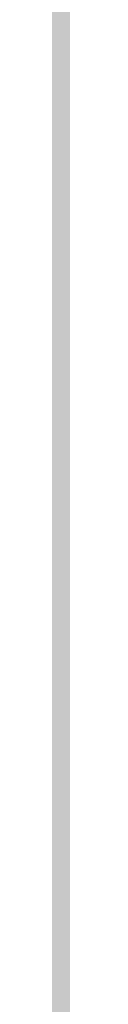
# Model space of a CAD drawing. Units: inches. Extents: x 2083 to 3317, y 1141 to 2115.
# Tile 218 of 256: x 3126.939 to 3126.956, y 1265.165 to 1267.234. Entities that reach past the tile are written whole.
import ezdxf

# ---------------------------------------------------------------- set-up
doc = ezdxf.new("R2010")
doc.units = ezdxf.units.IN
doc.layers.add('A-ANNO-DIMS', color=2, linetype='Continuous', lineweight=18)
doc.layers.add('A-WALL-PATT', color=251, linetype='Continuous', lineweight=13, true_color=0x636466)
doc.styles.get("Standard").update_dxf_attribs({"font": 'arial.ttf'})
doc.dimstyles.new('ISO-25', dxfattribs={"dimtxt": 12, "dimasz": 12, "dimexe": 1.25, "dimexo": 0.625, "dimtad": 1, "dimlunit": 3, "dimtxsty": 'Standard', "dimcen": 2.5, "dimadec": 0, "dimazin": 0, "dimtfac": 1, "dimtmove": 0, "dimatfit": 3, "dimfxl": 1, "dimarcsym": 0})

# ---------------------------------------------------------------- blocks, each defined once
blk = doc.blocks.new('*D26')
at = {"layer": 'A-ANNO-DIMS', "color": 0, "lineweight": -2, "transparency": 16777216}
for p, q in [((3088.9858, 1274.9151), (3088.9858, 1270.952)), ((3111.24, 1274.9151), (3111.24, 1270.952)), ((3076.9858, 1272.202), (2840.2624, 1272.202)), ((3111.24, 1272.202), (3088.9858, 1272.202)), ((3123.24, 1272.202), (3135.24, 1272.202))]:
    blk.add_line(p, q, dxfattribs=at)
at = {"layer": 'A-ANNO-DIMS', "color": 0, "transparency": 16777216}
for points in [[(3076.9858, 1274.202), (3076.9858, 1270.202), (3088.9858, 1272.202)], [(3123.24, 1274.202), (3123.24, 1270.202), (3111.24, 1272.202)]]:
    blk.add_solid(points, dxfattribs=at)
at = {"layer": 'Defpoints', "color": 0, "transparency": 16777216}
for p in [(3088.9858, 1275.5401), (3111.24, 1275.5401), (3088.9858, 1272.202)]:
    blk.add_point(p, dxfattribs=at)
at = {"layer": 'A-ANNO-DIMS', "color": 0, "transparency": 16777216, "insert": (2952.6241, 1279.0316), "char_height": 12, "attachment_point": 5}
blk.add_mtext('NIGHTSTAND 1\'-10 1/2" TYP.', dxfattribs=at)
blk = doc.blocks.new('*D27')
at = {"layer": 'A-ANNO-DIMS', "color": 0, "lineweight": -2, "transparency": 16777216}
for p, q in [((3114.5782, 1309.7943), (3114.5782, 1321.7943)), ((3111.865, 1297.7943), (3115.8282, 1297.7943)), ((3114.5782, 1297.7943), (3114.5782, 1275.5401)), ((3111.865, 1275.5401), (3115.8282, 1275.5401)), ((3114.5782, 1263.5401), (3114.5782, 1140.9886))]:
    blk.add_line(p, q, dxfattribs=at)
at = {"layer": 'A-ANNO-DIMS', "color": 0, "transparency": 16777216}
for points in [[(3112.5782, 1309.7943), (3116.5782, 1309.7943), (3114.5782, 1297.7943)], [(3112.5782, 1263.5401), (3116.5782, 1263.5401), (3114.5782, 1275.5401)]]:
    blk.add_solid(points, dxfattribs=at)
at = {"layer": 'Defpoints', "color": 0, "transparency": 16777216}
for p in [(3111.24, 1297.7943), (3111.24, 1275.5401), (3114.5782, 1275.5401)]:
    blk.add_point(p, dxfattribs=at)
at = {"layer": 'A-ANNO-DIMS', "color": 0, "transparency": 16777216, "insert": (3107.7485, 1196.2643), "char_height": 12, "attachment_point": 5, "rotation": 90}
blk.add_mtext('1\'-10 1/2" TYP.', dxfattribs=at)

msp = doc.modelspace()

# ---------------------------------------------------------------- hatches: boundary and pattern name
at = {"layer": 'A-WALL-PATT'}
h = msp.add_hatch(color=256, dxfattribs=at)
h.dxf.hatch_style = 1
h.paths.add_polyline_path([(3126.9598, 2020.7614), (2748.9598, 2020.7614), (2604.9598, 2020.7614), (2226.9598, 2020.7614), (2226.9598, 1702.7614), (2466.9598, 1702.7614), (2466.9598, 1582.7614), (2418.9598, 1582.7614), (2418.9598, 1477.7614), (2226.9598, 1477.7614), (2226.9598, 1263.2614), (2544.9598, 1263.2614), (2544.9598, 1411.7614), (2604.9598, 1411.7614), (2685.9598, 1411.7614), (2685.9598, 1420.7614), (2604.9598, 1420.7614), (2604.9598, 1573.7614), (2604.9598, 1702.7614), (2604.9598, 2011.7614), (2748.9598, 2011.7614), (2748.9598, 1702.7614), (2862.9598, 1702.7614), (2862.9598, 1621.7614), (2871.9598, 1621.7614), (2871.9598, 1702.7614), (2883.9598, 1702.7614), (2883.9598, 1706.9395, -0.026459), (2883.9598, 1711.7614), (2757.9598, 1711.7614), (2757.9598, 1807.7614), (2787.9598, 1807.7614), (2787.9598, 1812.2614), (2757.9598, 1812.2614), (2757.9598, 2011.7614), (2877.9598, 2011.7614), (2877.9598, 1812.2614), (2847.9598, 1812.2614), (2847.9598, 1807.7614), (2889.8357, 1807.7614), (2889.8357, 1812.2614), (2882.4598, 1812.2614), (2882.4598, 2011.7614), (3117.9598, 2011.7614), (3117.9598, 1812.2614), (2937.8357, 1812.2614), (2937.8357, 1807.7614), (2995.7098, 1807.7614), (2995.7098, 1796.1177), (3000.2098, 1796.1177), (3000.2098, 1807.7614), (3117.9598, 1807.7614), (3117.9598, 1711.7614), (3000.2098, 1711.7614), (3000.2098, 1760.1177), (2998.5727, 1760.1177, -0.020711), (2995.7098, 1760.1177), (2995.7098, 1711.7614), (2931.9598, 1711.7614), (2931.9598, 1702.7614), (3126.9598, 1702.7614)])
h.paths.add_polyline_path([(2471.4598, 2011.7614), (2471.4598, 1810.0114), (2462.7169, 1810.0114), (2462.7169, 1805.5114), (2505.9598, 1805.5114), (2505.9598, 1810.0114), (2475.9598, 1810.0114), (2475.9598, 2011.7614), (2595.9598, 2011.7614), (2595.9598, 1810.0114), (2565.9598, 1810.0114), (2565.9598, 1805.5114), (2595.9598, 1805.5114), (2595.9598, 1711.7614), (2235.9598, 1711.7614), (2235.9598, 1805.5114), (2353.7098, 1805.5114), (2353.7098, 1796.0542), (2358.2098, 1796.0542), (2358.2098, 1805.5114), (2414.7169, 1805.5114), (2414.7169, 1810.0114), (2235.9598, 1810.0114), (2235.9598, 2011.7614)], flags=16)
h.paths.add_polyline_path([(2270.2047, 1994.61), (2270.2047, 1970.61), (2246.2047, 1970.61), (2246.2047, 1994.61)], flags=0)
edge = h.paths.add_edge_path(flags=0)
edge.add_ellipse((2332.0274, 1899.7982), major_axis=(-3.043, 3.043), ratio=0.168252, start_angle=-161.3322, end_angle=-156.3071, ccw=False)
edge.add_ellipse((2333.082, 1898.7435), major_axis=(-1.0546, 1.0546), ratio=0.453532, start_angle=-123.371, end_angle=-94.1591)
edge = h.paths.add_edge_path(flags=0)
edge.add_ellipse((2332.0274, 1968.8763), major_axis=(3.043, 3.043), ratio=0.168252, start_angle=18.6678, end_angle=23.6929)
edge.add_spline(control_points=[(2332.9256, 1970.6911), (2332.2268, 1970.3361), (2330.8937, 1969.6589), (2328.4131, 1970.9321), (2327.2039, 1967.7487), (2324.7096, 1969.9556), (2322.5328, 1967.0124), (2320.0128, 1971.2958), (2317.6803, 1968.1578), (2316.0405, 1967.102), (2315.4269, 1966.8096)], knot_values=[0, 0, 0, 0, 2.267059, 4.324559, 6.685584, 8.878641, 11.121502, 14.300359, 17.755284, 19.732645, 19.732645, 19.732645, 19.732645], degree=3, periodic=0)
edge.add_ellipse((2332.0274, 1968.8763), major_axis=(3.043, 3.043), ratio=0.168252, start_angle=18.6678, end_angle=23.6929, ccw=False)
edge.add_ellipse((2333.082, 1969.9309), major_axis=(1.0546, 1.0546), ratio=0.453532, start_angle=56.629, end_angle=85.8409, ccw=False)
edge = h.paths.add_edge_path(flags=0)
edge.add_spline(control_points=[(2296.4283, 1967.9879), (2293.6278, 1965.3363), (2287.7036, 1959.7271), (2299.7439, 1949.9957), (2294.5326, 1935.6685), (2290.5732, 1920.6035), (2293.3941, 1909.9737), (2296.1854, 1904.9665)], knot_values=[0.099185, 0.099185, 0.099185, 0.099185, 0.345301, 0.619822, 0.982653, 1.386093, 1.810555, 1.810555, 1.810555, 1.810555], degree=3, periodic=0)
edge.add_spline(control_points=[(2296.1854, 1904.9665), (2297.3836, 1902.6193), (2298.001, 1901.9493), (2298.553, 1901.4682)], knot_values=[0.006246, 0.006246, 0.006246, 0.006246, 0.055476, 0.055476, 0.055476, 0.055476], degree=3, periodic=0)
edge.add_spline(control_points=[(2298.553, 1901.4682), (2297.2586, 1900.9232), (2295.2253, 1900.2321), (2293.0602, 1900.6142), (2292.1014, 1900.7884), (2292.0896, 1900.7906)], knot_values=[0.312835, 0.312835, 0.312835, 0.312835, 0.40178, 0.474987, 0.475903, 0.475903, 0.475903, 0.475903], degree=3, periodic=0)
edge.add_arc((2292.7936, 1904.6641), 3.937, 215.4209, 259.6982, ccw=False)
edge.add_spline(control_points=[(2289.5853, 1902.3823), (2289.4767, 1902.5351), (2289.3685, 1902.688), (2289.2609, 1902.8412)], knot_values=[0.102872, 0.102872, 0.102872, 0.102872, 0.116896, 0.116896, 0.116896, 0.116896], degree=3, periodic=0)
edge.add_spline(control_points=[(2289.2609, 1902.8412), (2288.6866, 1902.5502), (2287.64, 1902.0199), (2285.8813, 1901.874), (2283.853, 1901.5044), (2281.72, 1899.7105), (2278.467, 1899.4929), (2276.1571, 1901.8832), (2272.259, 1899.8041), (2267.7776, 1901.8432), (2262.2439, 1900.184), (2257.4149, 1901.7821), (2254.3184, 1900.7261), (2253.1783, 1900.3373)], knot_values=[0, 0, 0, 0, 1.907977, 3.477176, 5.261074, 7.972851, 11.680248, 13.717921, 16.939592, 22.789562, 27.502503, 33.595215, 37.145618, 37.145618, 37.145618, 37.145618], degree=3, periodic=0)
edge.add_line((2253.1783, 1900.3373), (2250.2442, 1902.8412))
edge.add_line((2250.2442, 1902.8412), (2250.2442, 1965.8333))
edge.add_line((2250.2442, 1965.8333), (2253.1783, 1968.3371))
edge.add_spline(control_points=[(2253.1783, 1968.3371), (2254.3184, 1967.9483), (2257.4149, 1966.8924), (2262.2439, 1968.4904), (2267.7776, 1966.8313), (2271.5267, 1968.5372), (2273.8759, 1967.8283), (2274.2067, 1967.7276)], knot_values=[0, 0, 0, 0, 0.09018, 0.244935, 0.364644, 0.513233, 0.537855, 0.537855, 0.537855, 0.537855], degree=3, periodic=0)
edge.add_arc((2274.3529, 1963.7933), 3.937, 72.0511, 92.1279, ccw=False)
edge.add_arc((2281.2969, 1985.23), 18.5963, 252.05113, 288.56572)
edge.add_arc((2292.3167, 1956.0289), 12.6461, 71.02679, 113.77822, ccw=False)
edge = h.paths.add_edge_path(flags=0)
edge.add_spline(control_points=[(2274.8994, 1951.8562), (2275.0662, 1951.6166), (2275.2327, 1951.3766), (2275.398, 1951.1359)], knot_values=[1.409916, 1.409916, 1.409916, 1.409916, 1.43159, 1.43159, 1.43159, 1.43159], degree=3, periodic=0)
edge.add_spline(control_points=[(2275.398, 1951.1359), (2275.7921, 1950.5619), (2276.1792, 1949.9838), (2276.5455, 1949.3971)], knot_values=[1.358238, 1.358238, 1.358238, 1.358238, 1.409916, 1.409916, 1.409916, 1.409916], degree=3, periodic=0)
edge.add_line((2276.5455, 1949.3971), (2277.4373, 1947.8622))
edge.add_spline(control_points=[(2277.4373, 1947.8622), (2276.3038, 1945.6731), (2274.6397, 1942.4269), (2274.6316, 1938.0939), (2272.7991, 1930.8515), (2274.3564, 1943.897), (2275.9477, 1947.9234), (2276.5455, 1949.3971)], knot_values=[0.005632, 0.005632, 0.005632, 0.005632, 0.186014, 0.266002, 0.357087, 0.59639, 0.739732, 0.739732, 0.739732, 0.739732], degree=3, periodic=0)
edge.add_spline(control_points=[(2276.5455, 1949.3971), (2276.1792, 1949.9838), (2275.7921, 1950.5619), (2275.398, 1951.1359)], knot_values=[1.358238, 1.358238, 1.358238, 1.358238, 1.409916, 1.409916, 1.409916, 1.409916], degree=3, periodic=0)
edge.add_spline(control_points=[(2275.398, 1951.1359), (2274.9425, 1950.0805), (2274.2078, 1948.0253), (2273.9346, 1944.8515), (2272.4685, 1937.6275), (2273.4662, 1945.6965), (2274.7006, 1951.0595), (2274.8994, 1951.8562)], knot_values=[0.104364, 0.104364, 0.104364, 0.104364, 0.189636, 0.269624, 0.36071, 0.600013, 0.644622, 0.644622, 0.644622, 0.644622], degree=3, periodic=0)
h.paths.add_polyline_path([(2269.1675, 1963.1276, -0.357527), (2268.1706, 1960.9764, -0.092561), (2268.1706, 1939.4363, -0.357527), (2269.1675, 1937.2851, -0.357527), (2267.0163, 1938.282, -0.164785), (2254.6856, 1938.282, -0.357527), (2252.5344, 1937.2851, -0.357527), (2253.5313, 1939.4363, -0.092561), (2253.5313, 1960.9764, -0.357527), (2252.5344, 1963.1276, -0.357527), (2254.6856, 1962.1307, -0.164785), (2267.0163, 1962.1307, -0.357527)], flags=0)
h.paths.add_polyline_path([(2248.8741, 1967.8018), (2248.8741, 1957.0277), (2249.4578, 1957.0277), (2249.4578, 1911.6468), (2248.8741, 1911.6468), (2248.8741, 1900.8727), (2246.5119, 1900.8727, 0.197327), (2244.1497, 1902.4569), (2244.1497, 1966.2176, 0.197327), (2246.5119, 1967.8018)], flags=0)
h.paths.add_polyline_path([(2269.1675, 1931.3893, -0.357527), (2268.1706, 1929.2381, -0.092561), (2268.1706, 1907.6981, -0.357527), (2269.1675, 1905.5469, -0.357527), (2267.0163, 1906.5438, -0.164785), (2254.6856, 1906.5438, -0.357527), (2252.5344, 1905.5469, -0.357527), (2253.5313, 1907.6981, -0.092561), (2253.5313, 1929.2381, -0.357527), (2252.5344, 1931.3893, -0.357527), (2254.6856, 1930.3925, -0.164785), (2267.0163, 1930.3925, -0.357527)], flags=0)
edge = h.paths.add_edge_path(flags=0)
edge.add_spline(control_points=[(2276.1969, 1906.7237), (2276.1681, 1909.0289), (2276.114, 1913.3719), (2270.5984, 1924.925), (2273.9052, 1919.0128), (2275.9217, 1916.2621), (2275.4746, 1912.4021), (2277.2579, 1910.3806), (2276.696, 1908.225), (2276.6462, 1906.813), (2276.6178, 1906.0084)], knot_values=[0, 0, 0, 0, 8.61026, 16.221274, 18.843057, 23.804898, 27.440828, 29.356102, 31.203478, 33.650687, 33.650687, 33.650687, 33.650687], degree=3, periodic=0)
edge.add_spline(control_points=[(2276.6178, 1906.0084), (2276.6233, 1905.6241), (2276.4977, 1904.6287), (2275.4418, 1903.8547), (2274.9373, 1903.0804), (2274.8591, 1902.8412)], knot_values=[0.156488, 0.156488, 0.156488, 0.156488, 0.184398, 0.231376, 0.250598, 0.250598, 0.250598, 0.250598], degree=3, periodic=0)
edge.add_line((2274.8591, 1902.8412), (2276.506, 1902.8412))
edge.add_spline(control_points=[(2276.506, 1902.8412), (2276.7883, 1903.0849), (2277.6651, 1904.1252), (2278.2495, 1904.3407), (2277.6539, 1908.5274), (2278.1557, 1906.2278), (2278.1005, 1905.2859), (2278.8467, 1904.069), (2277.8568, 1903.4149), (2277.8742, 1902.991), (2277.9036, 1902.8412)], knot_values=[0.059574, 0.059574, 0.059574, 0.059574, 0.080753, 0.103741, 0.16972, 0.176036, 0.207137, 0.240474, 0.262341, 0.27366, 0.27366, 0.27366, 0.27366], degree=3, periodic=0)
edge.add_line((2277.9036, 1902.8412), (2280.0298, 1902.8412))
edge.add_spline(control_points=[(2280.0298, 1902.8412), (2279.8882, 1903.0884), (2279.4993, 1903.9816), (2280.1523, 1905.9393), (2278.1036, 1909.6578), (2279.7624, 1907.1853), (2280.3279, 1904.8749), (2280.4851, 1903.4896), (2281.4633, 1903.2494), (2281.7583, 1902.9365), (2281.834, 1902.8412)], knot_values=[0.013856, 0.013856, 0.013856, 0.013856, 0.034874, 0.088867, 0.107879, 0.126738, 0.158714, 0.193757, 0.217487, 0.226722, 0.226722, 0.226722, 0.226722], degree=3, periodic=0)
edge.add_spline(control_points=[(2281.834, 1902.8412), (2281.7875, 1902.8267), (2281.647, 1902.783), (2281.3955, 1902.8595), (2281.0881, 1902.9852), (2280.7207, 1903.0609), (2280.3335, 1903.0257), (2280.1248, 1902.8989), (2280.0298, 1902.8412)], knot_values=[0, 0, 0, 0, 0.14413, 0.435517, 0.749276, 1.153046, 1.548371, 1.878348, 1.878348, 1.878348, 1.878348], degree=3, periodic=0)
edge.add_line((2280.0298, 1902.8412), (2277.9036, 1902.8412))
edge.add_spline(control_points=[(2277.9036, 1902.8412), (2277.8929, 1902.7959), (2277.8654, 1902.6796), (2277.6075, 1902.6875), (2277.2741, 1902.8007), (2276.8379, 1902.6198), (2276.5838, 1902.7893), (2276.506, 1902.8412)], knot_values=[0, 0, 0, 0, 0.127189, 0.326199, 0.628009, 1.24357, 1.515331, 1.515331, 1.515331, 1.515331], degree=3, periodic=0)
edge.add_line((2276.506, 1902.8412), (2274.8591, 1902.8412))
edge.add_spline(control_points=[(2274.8591, 1902.8412), (2274.8144, 1902.8986), (2274.7251, 1903.0134), (2274.4935, 1903.119), (2274.2443, 1902.9605), (2273.9371, 1903.1849), (2273.614, 1902.9831), (2273.4083, 1902.883), (2273.3223, 1902.8412)], knot_values=[0, 0, 0, 0, 0.21843, 0.436957, 0.687977, 0.990379, 1.398396, 1.69185, 1.69185, 1.69185, 1.69185], degree=3, periodic=0)
edge.add_spline(control_points=[(2273.3223, 1902.8412), (2273.6167, 1903.4457), (2274.274, 1904.5383), (2276.0272, 1904.5737), (2276.207, 1906.5836), (2276.1969, 1906.7237)], knot_values=[0.012227, 0.012227, 0.012227, 0.012227, 0.059472, 0.106218, 0.134458, 0.134458, 0.134458, 0.134458], degree=3, periodic=0)
h.paths.add_polyline_path([(2270.7761, 1897.7898), (2270.7761, 1873.7898), (2246.7761, 1873.7898), (2246.7761, 1897.7898)], flags=0)
h.paths.add_polyline_path([(2353.7098, 1760.0051), (2353.7098, 1760.0542), (2358.2098, 1760.0542, -0.033729)], flags=0)
h.paths.add_polyline_path([(2321.8191, 1737.5292), (2341.9953, 1737.5292, -0.414214), (2343.2033, 1736.3212), (2343.2033, 1721.0206, -0.414214), (2341.9953, 1719.8127), (2321.8191, 1719.8127, -0.414214), (2320.6112, 1721.0206), (2320.6112, 1736.3212, -0.414214)], flags=0)
h.paths.add_polyline_path([(2324.235, 1736.3212), (2339.5794, 1736.3212, -0.414214), (2341.9953, 1733.9053), (2341.9953, 1725.4497, -0.414214), (2339.5794, 1723.0338), (2333.6806, 1723.0338), (2333.8453, 1722.0455, -0.870646), (2335.4254, 1721.8259, -0.767327), (2333.9227, 1721.4232), (2331.291, 1721.4232, -0.767327), (2329.7883, 1721.8259, -0.870646), (2331.3684, 1722.0455), (2331.5331, 1723.0338), (2324.235, 1723.0338, -0.414214), (2321.8191, 1725.4497), (2321.8191, 1733.9053, -0.414214)], flags=0)
h.paths.add_polyline_path([(2570.4838, 1928.6154), (2589.6838, 1928.6154), (2590.1688, 1928.6154), (2590.1688, 1904.9934), (2570.4838, 1904.9934)], flags=0)
h.paths.add_polyline_path([(2574.4473, 1927.2638, -1), (2572.8288, 1927.2638, -1)], flags=0)
h.paths.add_polyline_path([(2573.0899, 1926.9409), (2573.925, 1927.776), (2574.1477, 1927.5533), (2573.3126, 1926.7182)], flags=0)
h.paths.add_polyline_path([(2578.7791, 1919.7296, -1), (2571.5917, 1919.7296, -1)], flags=0)
h.paths.add_polyline_path([(2578.3854, 1919.7296, -1), (2571.9854, 1919.7296, -1)], flags=0)
h.paths.add_polyline_path([(2331.5958, 1729.4762, -1), (2333.618, 1729.4762, -1)], flags=0)
h.paths.add_polyline_path([(2578.0342, 1927.2638, -1), (2576.4157, 1927.2638, -1)], flags=0)
h.paths.add_polyline_path([(2576.6889, 1927.5311), (2576.9116, 1927.7538), (2577.7467, 1926.9186), (2577.524, 1926.6959)], flags=0)
h.paths.add_polyline_path([(2578.1391, 1909.8595, -1), (2572.2317, 1909.8595, -1)], flags=0)
h.paths.add_polyline_path([(2577.7454, 1909.8595, -1), (2572.6254, 1909.8595, -1)], flags=0)
h.paths.add_polyline_path([(2583.7977, 1927.2638, -1), (2582.1792, 1927.2638, -1)], flags=0)
h.paths.add_polyline_path([(2582.7186, 1927.7538), (2583.5538, 1926.9186), (2583.3311, 1926.6959), (2582.4959, 1927.5311)], flags=0)
h.paths.add_polyline_path([(2582.4959, 1927.5311), (2582.7186, 1927.7538), (2583.5538, 1926.9186), (2583.3311, 1926.6959)], flags=0)
h.paths.add_polyline_path([(2587.7391, 1920.5296, -1), (2581.8317, 1920.5296, -1)], flags=0)
h.paths.add_polyline_path([(2587.3454, 1920.5296, -1), (2582.2254, 1920.5296, -1)], flags=0)
h.paths.add_polyline_path([(2587.3846, 1927.2638, -1), (2585.7661, 1927.2638, -1)], flags=0)
h.paths.add_polyline_path([(2586.082, 1926.9802), (2586.9172, 1927.8154), (2587.1399, 1927.5927), (2586.3047, 1926.7575)], flags=0)
h.paths.add_polyline_path([(2588.3791, 1910.6595, -1), (2581.1917, 1910.6595, -1)], flags=0)
h.paths.add_polyline_path([(2587.9854, 1910.6595, -1), (2581.5854, 1910.6595, -1)], flags=0)
h.paths.add_polyline_path([(2417.1677, 1729.4779), (2437.3439, 1729.4779, -0.414214), (2438.5519, 1728.2699), (2438.5519, 1712.9693, -0.414214), (2437.3439, 1711.7614), (2417.1677, 1711.7614, -0.414214), (2415.9598, 1712.9693), (2415.9598, 1728.2699, -0.414214)], flags=0)
h.paths.add_polyline_path([(2419.5836, 1728.2699), (2434.928, 1728.2699, -0.414214), (2437.3439, 1725.8541), (2437.3439, 1717.3984, -0.414214), (2434.928, 1714.9825), (2429.0292, 1714.9825), (2429.1939, 1713.9942, -0.870646), (2430.774, 1713.7746, -0.767327), (2429.2713, 1713.372), (2426.6396, 1713.372, -0.767327), (2425.1369, 1713.7746, -0.870646), (2426.717, 1713.9942), (2426.8817, 1714.9825), (2419.5836, 1714.9825, -0.414214), (2417.1677, 1717.3984), (2417.1677, 1725.8541, -0.414214)], flags=0)
h.paths.add_polyline_path([(2419.5836, 1728.2699), (2434.928, 1728.2699, -0.414214), (2437.3439, 1725.8541), (2437.3439, 1717.3984, -0.414214), (2434.928, 1714.9825), (2429.0292, 1714.9825), (2428.3581, 1719.009), (2427.5528, 1719.009), (2426.8817, 1714.9825), (2419.5836, 1714.9825, -0.414214), (2417.1677, 1717.3984), (2417.1677, 1725.8541, -0.414214)], flags=0)
h.paths.add_polyline_path([(2426.9444, 1721.4249, -1), (2428.9666, 1721.4249, -1)], flags=0)
h.paths.add_polyline_path([(2475.9598, 1702.7614), (2595.9598, 1702.7614), (2595.9598, 1582.7614), (2475.9598, 1582.7614)], flags=16)
h.paths.add_polyline_path([(2427.9598, 1573.7614), (2595.9598, 1573.7614), (2595.9598, 1468.7614), (2595.9598, 1420.7614), (2384.4598, 1420.7614), (2384.4598, 1468.7614), (2427.9598, 1468.7614)], flags=16)
h.paths.add_polyline_path([(2379.9598, 1468.7614), (2379.9598, 1420.7614), (2235.9598, 1420.7614), (2235.9598, 1468.7614)], flags=16)
h.paths.add_polyline_path([(2317.816, 1466.6958), (2337.9922, 1466.6958, -0.414214), (2339.2002, 1465.4878), (2339.2002, 1450.1872, -0.414214), (2337.9922, 1448.9792), (2317.816, 1448.9792, -0.414214), (2316.6081, 1450.1872), (2316.6081, 1465.4878, -0.414214)], flags=0)
h.paths.add_polyline_path([(2320.2319, 1465.4878), (2335.5763, 1465.4878, -0.414214), (2337.9922, 1463.0719), (2337.9922, 1454.6163, -0.414214), (2335.5763, 1452.2004), (2329.6775, 1452.2004), (2329.8422, 1451.212, -0.870646), (2331.4223, 1450.9925, -0.767327), (2329.9196, 1450.5898), (2327.2879, 1450.5898, -0.767327), (2325.7852, 1450.9925, -0.870646), (2327.3653, 1451.212), (2327.53, 1452.2004), (2320.2319, 1452.2004, -0.414214), (2317.816, 1454.6163), (2317.816, 1463.0719, -0.414214)], flags=0)
h.paths.add_polyline_path([(2320.2319, 1465.4878), (2335.5763, 1465.4878, -0.414214), (2337.9922, 1463.0719), (2337.9922, 1454.6163, -0.414214), (2335.5763, 1452.2004), (2329.6775, 1452.2004), (2329.0064, 1456.2269), (2328.2011, 1456.2269), (2327.53, 1452.2004), (2320.2319, 1452.2004, -0.414214), (2317.816, 1454.6163), (2317.816, 1463.0719, -0.414214)], flags=0)
h.paths.add_polyline_path([(2327.5926, 1458.6428, -1), (2329.6148, 1458.6428, -1)], flags=0)
h.paths.add_polyline_path([(2244.4117, 1433.3405), (2241.9209, 1433.3405, -0.414214), (2240.0179, 1435.2435), (2240.0179, 1440.9528, -0.414211), (2241.9209, 1442.8559), (2244.4117, 1442.8559, -1.976472)], flags=0)
h.paths.add_polyline_path([(2245.3569, 1434.3975, -0.414214), (2245.3569, 1441.7988, -2.144098)], flags=0)
h.paths.add_polyline_path([(2535.9598, 1416.2614), (2535.9598, 1272.2614), (2235.9598, 1272.2614), (2235.9598, 1416.2614)], flags=16)
h.paths.add_polyline_path([(2260.1196, 1384.2928), (2260.1196, 1362.0386), (2237.8654, 1362.0386), (2237.8654, 1384.2928)], flags=0)
edge = h.paths.add_edge_path(flags=0)
edge.add_line((2318.2518, 1362.0933), (2318.1458, 1362.001))
edge.add_ellipse((2317.4451, 1360.431), major_axis=(2.8216, 2.8216), ratio=0.168252, start_angle=18.6678, end_angle=20.9481, ccw=False)
edge.add_ellipse((2318.423, 1361.409), major_axis=(0.9779, 0.9779), ratio=0.453532, start_angle=56.629, end_angle=70.2262, ccw=False)
edge = h.paths.add_edge_path(flags=0)
edge.add_line((2319.1074, 1295.5711), (2319.015, 1295.6771))
edge.add_ellipse((2317.4451, 1296.3778), major_axis=(-2.8216, 2.8216), ratio=0.168252, start_angle=-161.3322, end_angle=-159.0519, ccw=False)
edge.add_ellipse((2318.423, 1295.3999), major_axis=(-0.9779, 0.9779), ratio=0.453532, start_angle=-123.371, end_angle=-109.7738)
edge = h.paths.add_edge_path(flags=0)
edge.add_spline(control_points=[(2284.2103, 1301.1702), (2284.5807, 1300.4447), (2284.8912, 1299.892), (2285.1596, 1299.461)], knot_values=[0.039066, 0.039066, 0.039066, 0.039066, 0.055476, 0.055476, 0.055476, 0.055476], degree=3, periodic=0)
edge.add_line((2285.1596, 1299.461), (2284.2103, 1301.1702))
edge = h.paths.add_edge_path(flags=0)
edge.add_line((2280.4125, 1297.298), (2283.37, 1297.0361))
edge.add_line((2283.37, 1297.0361), (2286.4057, 1297.9263))
edge.add_spline(control_points=[(2286.4057, 1297.9263), (2285.3055, 1297.4631), (2284.3448, 1297.1292), (2283.37, 1297.0361)], knot_values=[0.394369, 0.394369, 0.394369, 0.394369, 0.475903, 0.475903, 0.475903, 0.475903], degree=3, periodic=0)
edge.add_spline(control_points=[(2283.37, 1297.0361), (2283.2814, 1297.0277), (2282.3163, 1296.9573), (2281.3125, 1297.1345), (2280.4234, 1297.296), (2280.4125, 1297.298)], knot_values=[0.312835, 0.312835, 0.312835, 0.312835, 0.320246, 0.393453, 0.394369, 0.394369, 0.394369, 0.394369], degree=3, periodic=0)
edge = h.paths.add_edge_path(flags=0)
edge.add_line((2284.4356, 1359.6073), (2280.4463, 1355.328))
edge.add_line((2280.4463, 1355.328), (2279.58, 1351.0178))
edge.add_line((2279.58, 1351.0178), (2282.413, 1346.5804))
edge.add_spline(control_points=[(2282.413, 1346.5804), (2283.1533, 1345.5892), (2284.2529, 1344.0289), (2284.801, 1342.3872), (2284.9352, 1341.8055)], knot_values=[1.240098, 1.240098, 1.240098, 1.240098, 1.332892, 1.382712, 1.382712, 1.382712, 1.382712], degree=3, periodic=0)
edge.add_spline(control_points=[(2284.9352, 1341.8055), (2285.3191, 1340.1406), (2285.233, 1338.4092), (2284.9099, 1336.6541)], knot_values=[1.097484, 1.097484, 1.097484, 1.097484, 1.240098, 1.240098, 1.240098, 1.240098], degree=3, periodic=0)
edge.add_spline(control_points=[(2284.9099, 1336.6541), (2284.5868, 1334.899), (2284.0267, 1333.1203), (2283.4626, 1331.3606)], knot_values=[0.95487, 0.95487, 0.95487, 0.95487, 1.097484, 1.097484, 1.097484, 1.097484], degree=3, periodic=0)
edge.add_line((2283.4626, 1331.3606), (2281.8904, 1326.1534))
edge.add_line((2281.8904, 1326.1534), (2280.7563, 1321.0561))
edge.add_line((2280.7563, 1321.0561), (2280.2992, 1316.002))
edge.add_line((2280.2992, 1316.002), (2280.7159, 1310.9501))
edge.add_line((2280.7159, 1310.9501), (2282.0281, 1305.9721))
edge.add_line((2282.0281, 1305.9721), (2284.2103, 1301.1702))
edge.add_spline(control_points=[(2284.2103, 1301.1702), (2283.3407, 1302.7302), (2282.6119, 1304.3365), (2282.0281, 1305.9721)], knot_values=[0.099185, 0.099185, 0.099185, 0.099185, 0.241799, 0.241799, 0.241799, 0.241799], degree=3, periodic=0)
edge.add_spline(control_points=[(2282.0281, 1305.9721), (2281.4443, 1307.6078), (2281.0055, 1309.2728), (2280.7159, 1310.9501)], knot_values=[0.241799, 0.241799, 0.241799, 0.241799, 0.384413, 0.384413, 0.384413, 0.384413], degree=3, periodic=0)
edge.add_spline(control_points=[(2280.7159, 1310.9501), (2280.4332, 1312.5876), (2280.2894, 1314.277), (2280.2989, 1315.962), (2280.2992, 1316.002)], knot_values=[0.384413, 0.384413, 0.384413, 0.384413, 0.523647, 0.527028, 0.527028, 0.527028, 0.527028], degree=3, periodic=0)
edge.add_spline(control_points=[(2280.2992, 1316.002), (2280.3123, 1317.687), (2280.4779, 1319.3679), (2280.7563, 1321.0561)], knot_values=[0.527028, 0.527028, 0.527028, 0.527028, 0.669642, 0.669642, 0.669642, 0.669642], degree=3, periodic=0)
edge.add_spline(control_points=[(2280.7563, 1321.0561), (2281.0346, 1322.7443), (2281.4259, 1324.4396), (2281.8904, 1326.1534)], knot_values=[0.669642, 0.669642, 0.669642, 0.669642, 0.812256, 0.812256, 0.812256, 0.812256], degree=3, periodic=0)
edge.add_spline(control_points=[(2281.8904, 1326.1534), (2282.2644, 1327.5333), (2282.7879, 1329.2618), (2283.3528, 1331.0178), (2283.4626, 1331.3606)], knot_values=[0.812256, 0.812256, 0.812256, 0.812256, 0.927087, 0.95487, 0.95487, 0.95487, 0.95487], degree=3, periodic=0)
edge.add_line((2283.4626, 1331.3606), (2284.9099, 1336.6541))
edge.add_line((2284.9099, 1336.6541), (2284.9352, 1341.8055))
edge.add_line((2284.9352, 1341.8055), (2282.413, 1346.5804))
edge.add_spline(control_points=[(2282.413, 1346.5804), (2281.2751, 1348.1038), (2280.0784, 1349.5703), (2279.58, 1351.0178)], knot_values=[1.382712, 1.382712, 1.382712, 1.382712, 1.525326, 1.525326, 1.525326, 1.525326], degree=3, periodic=0)
edge.add_spline(control_points=[(2279.58, 1351.0178), (2279.4433, 1351.4147), (2279.1363, 1352.8569), (2279.7352, 1354.2904), (2280.4463, 1355.328)], knot_values=[1.525326, 1.525326, 1.525326, 1.525326, 1.564439, 1.667941, 1.667941, 1.667941, 1.667941], degree=3, periodic=0)
edge.add_spline(control_points=[(2280.4463, 1355.328), (2281.4261, 1356.7578), (2282.9308, 1358.1826), (2284.4356, 1359.6073)], knot_values=[1.667941, 1.667941, 1.667941, 1.667941, 1.810555, 1.810555, 1.810555, 1.810555], degree=3, periodic=0)
edge.add_arc((2280.6231, 1348.5182), 11.7262, 71.02679, 113.77822)
edge.add_arc((2270.4049, 1375.5952), 17.2436, 252.05113, 288.56572, ccw=False)
edge.add_arc((2263.966, 1355.7178), 3.6506, 72.0511, 92.1279)
edge.add_arc((2263.966, 1355.7178), 3.6506, 92.1279, 177.9851)
edge.add_spline(control_points=[(2260.3176, 1355.8462), (2260.2604, 1354.2207), (2260.5513, 1350.1865), (2262.9993, 1346.7663), (2264.4727, 1344.649)], knot_values=[1.43159, 1.43159, 1.43159, 1.43159, 1.564144, 1.770695, 1.770695, 1.770695, 1.770695], degree=3, periodic=0)
edge.add_line((2264.4727, 1344.649), (2264.9356, 1343.9825))
edge.add_spline(control_points=[(2263.801, 1340.2481), (2263.8432, 1340.5141), (2264.0672, 1341.7565), (2264.5127, 1343.0025), (2264.935, 1343.9811)], knot_values=[0.53657, 0.53657, 0.53657, 0.53657, 0.559349, 0.644622, 0.644622, 0.644622, 0.644622], degree=3, periodic=0)
edge.add_spline(control_points=[(2264.935, 1343.9811), (2265.1178, 1343.715), (2265.2989, 1343.4479), (2265.4768, 1343.1794)], knot_values=[1.384077, 1.384077, 1.384077, 1.384077, 1.409916, 1.409916, 1.409916, 1.409916], degree=3, periodic=0)
edge.add_spline(control_points=[(2265.4768, 1343.1794), (2265.6546, 1342.9108), (2265.8293, 1342.6408), (2265.9991, 1342.3688)], knot_values=[1.358238, 1.358238, 1.358238, 1.358238, 1.384077, 1.384077, 1.384077, 1.384077], degree=3, periodic=0)
edge.add_line((2265.9991, 1342.3688), (2266.826, 1340.9455))
edge.add_spline(control_points=[(2266.826, 1340.9455), (2268.8944, 1337.0897), (2271.3982, 1325.843), (2270.5162, 1310.5686), (2275.9194, 1301.8606), (2277.7895, 1299.1994)], knot_values=[0.116896, 0.116896, 0.116896, 0.116896, 0.472987, 1.050969, 1.313793, 1.313793, 1.313793, 1.313793], degree=3, periodic=0)
edge.add_spline(control_points=[(2277.7895, 1299.1994), (2277.8394, 1299.1285), (2277.8894, 1299.0575), (2277.9396, 1298.9866)], knot_values=[0.109884, 0.109884, 0.109884, 0.109884, 0.116896, 0.116896, 0.116896, 0.116896], degree=3, periodic=0)
edge.add_line((2277.9396, 1298.9866), (2277.7888, 1299.1991))
edge.add_spline(control_points=[(2277.7888, 1299.1991), (2277.2566, 1298.9294), (2276.2864, 1298.4379), (2275.0394, 1298.3344), (2274.3833, 1298.2389), (2274.2153, 1298.2093)], knot_values=[33.12187, 33.12187, 33.12187, 33.12187, 35.029056, 36.598255, 37.144827, 37.144827, 37.144827, 37.144827], degree=3, periodic=0)
edge.add_line((2274.2153, 1298.2093), (2273.0731, 1297.893))
edge.add_spline(control_points=[(2273.0731, 1297.893), (2272.3229, 1297.5798), (2271.0392, 1296.5105), (2269.2484, 1296.2261), (2268.4231, 1296.3747)], knot_values=[26.532584, 26.532584, 26.532584, 26.532584, 29.198919, 31.839101, 31.839101, 31.839101, 31.839101], degree=3, periodic=0)
edge.add_line((2268.4231, 1296.3747), (2263.8785, 1297.4575))
edge.add_spline(control_points=[(2263.8785, 1297.4575), (2263.5561, 1297.3594), (2261.8603, 1296.8387), (2260.2388, 1297.2824), (2258.9335, 1297.5165)], knot_values=[15.919551, 15.919551, 15.919551, 15.919551, 16.939592, 21.226067, 21.226067, 21.226067, 21.226067], degree=3, periodic=0)
edge.add_line((2258.9335, 1297.5165), (2254.0552, 1297.329))
edge.add_spline(control_points=[(2254.0552, 1297.329), (2253.7555, 1297.2958), (2252.1137, 1297.1652), (2250.4619, 1297.5442), (2249.1297, 1297.6679)], knot_values=[5.306517, 5.306517, 5.306517, 5.306517, 6.276435, 10.613034, 10.613034, 10.613034, 10.613034], degree=3, periodic=0)
edge.add_line((2249.1297, 1297.6679), (2244.3316, 1296.8778))
edge.add_line((2244.3316, 1296.8778), (2241.611, 1299.1994))
edge.add_line((2241.611, 1299.1994), (2241.611, 1357.6094))
edge.add_line((2241.611, 1357.6094), (2244.3316, 1359.9311))
edge.add_line((2244.3316, 1359.9311), (2252.7288, 1359.5427))
edge.add_spline(control_points=[(2252.7288, 1359.5427), (2252.8709, 1359.5464), (2253.3057, 1359.5482), (2253.7398, 1359.5143), (2254.0317, 1359.4824)], knot_values=[0.233291, 0.233291, 0.233291, 0.233291, 0.244935, 0.268927, 0.268927, 0.268927, 0.268927], degree=3, periodic=0)
edge.add_line((2254.0317, 1359.4824), (2259.5872, 1359.4164))
edge.add_spline(control_points=[(2259.5872, 1359.4164), (2260.6771, 1359.6285), (2262.0732, 1359.897), (2263.5237, 1359.4593), (2263.8304, 1359.366)], knot_values=[0.422516, 0.422516, 0.422516, 0.422516, 0.513233, 0.537855, 0.537855, 0.537855, 0.537855], degree=3, periodic=0)
edge.add_arc((2263.966, 1355.7178), 3.6506, 72.0511, 92.1279, ccw=False)
edge.add_arc((2270.4049, 1375.5952), 17.2436, 252.05113, 288.56572)
edge.add_arc((2280.6231, 1348.5182), 11.7262, 71.02679, 113.77822, ccw=False)
h.paths.add_polyline_path([(2240.3405, 1359.4347), (2240.3405, 1349.4444), (2240.8818, 1349.4444), (2240.8818, 1307.3645), (2240.3405, 1307.3645), (2240.3405, 1297.3741), (2238.1502, 1297.3741, 0.197327), (2235.9598, 1298.8431), (2235.9598, 1357.9657, 0.197327), (2238.1502, 1359.4347)], flags=0)
h.paths.add_polyline_path([(2259.1578, 1355.1005, -0.357527), (2258.2334, 1353.1058, -0.092561), (2258.2334, 1333.1326, -0.357527), (2259.1578, 1331.1379, -0.357527), (2257.1631, 1332.0622, -0.164785), (2245.7293, 1332.0622, -0.357527), (2243.7346, 1331.1379, -0.357527), (2244.6589, 1333.1326, -0.092561), (2244.6589, 1353.1058, -0.357527), (2243.7346, 1355.1005, -0.357527), (2245.7293, 1354.1761, -0.164785), (2257.1631, 1354.1761, -0.357527)], flags=0)
edge = h.paths.add_edge_path(flags=0)
edge.add_line((2265.9991, 1342.3688), (2266.826, 1340.9455))
edge.add_line((2266.826, 1340.9455), (2265.3076, 1337.8141))
edge.add_line((2265.3076, 1337.8141), (2264.3582, 1334.6529))
edge.add_line((2264.3582, 1334.6529), (2264.262, 1333.7997))
edge.add_spline(control_points=[(2264.262, 1333.7997), (2264.2084, 1333.1871), (2264.1621, 1332.3655), (2264.0071, 1331.4139), (2263.969, 1331.2018)], knot_values=[0.464444, 0.464444, 0.464444, 0.464444, 0.516691, 0.531608, 0.531608, 0.531608, 0.531608], degree=3, periodic=0)
edge.add_spline(control_points=[(2263.969, 1331.2018), (2263.7745, 1330.1189), (2263.4244, 1328.7908), (2263.2574, 1328.5307), (2263.234, 1328.5146)], knot_values=[0.372682, 0.372682, 0.372682, 0.372682, 0.44885, 0.464444, 0.464444, 0.464444, 0.464444], degree=3, periodic=0)
edge.add_spline(control_points=[(2263.234, 1328.5146), (2263.0964, 1328.4202), (2263.1312, 1329.3015), (2263.275, 1330.6157)], knot_values=[0.280919, 0.280919, 0.280919, 0.280919, 0.372682, 0.372682, 0.372682, 0.372682], degree=3, periodic=0)
edge.add_spline(control_points=[(2263.275, 1330.6157), (2263.4187, 1331.93), (2263.6715, 1333.6773), (2263.9699, 1335.315)], knot_values=[0.189157, 0.189157, 0.189157, 0.189157, 0.280919, 0.280919, 0.280919, 0.280919], degree=3, periodic=0)
edge.add_spline(control_points=[(2263.9699, 1335.315), (2264.1005, 1336.0322), (2264.4188, 1337.6219), (2264.7548, 1338.8644), (2264.9474, 1339.4911)], knot_values=[0.097394, 0.097394, 0.097394, 0.097394, 0.137578, 0.189157, 0.189157, 0.189157, 0.189157], degree=3, periodic=0)
edge.add_spline(control_points=[(2264.9474, 1339.4911), (2265.29, 1340.6061), (2265.6442, 1341.494), (2265.9991, 1342.3688)], knot_values=[0.005632, 0.005632, 0.005632, 0.005632, 0.097394, 0.097394, 0.097394, 0.097394], degree=3, periodic=0)
h.paths.add_polyline_path([(2259.1578, 1325.671, -0.357527), (2258.2334, 1323.6763, -0.092561), (2258.2334, 1303.7031, -0.357527), (2259.1578, 1301.7084, -0.357527), (2257.1631, 1302.6327, -0.164785), (2245.7293, 1302.6327, -0.357527), (2243.7346, 1301.7084, -0.357527), (2244.6589, 1303.7031, -0.092561), (2244.6589, 1323.6763, -0.357527), (2243.7346, 1325.671, -0.357527), (2245.7293, 1324.7466, -0.164785), (2257.1631, 1324.7466, -0.357527)], flags=0)
edge = h.paths.add_edge_path(flags=0)
edge.add_spline(control_points=[(2261.7089, 1317.3114), (2261.6795, 1317.4176), (2261.7619, 1317.3885), (2262.4907, 1316.0899), (2262.9622, 1315.3009)], knot_values=[14.955861, 14.955861, 14.955861, 14.955861, 16.221274, 18.694826, 18.694826, 18.694826, 18.694826], degree=3, periodic=0)
edge.add_spline(control_points=[(2262.9622, 1315.3009), (2262.9904, 1315.2536), (2263.7021, 1314.0674), (2264.349, 1313.1272), (2264.7301, 1312.1642)], knot_values=[18.694826, 18.694826, 18.694826, 18.694826, 18.843057, 22.433791, 22.433791, 22.433791, 22.433791], degree=3, periodic=0)
edge.add_spline(control_points=[(2264.7301, 1312.1642), (2264.8756, 1311.7964), (2265.1769, 1310.7698), (2265.1431, 1309.5593), (2265.2477, 1308.8242)], knot_values=[22.433791, 22.433791, 22.433791, 22.433791, 23.804898, 26.172756, 26.172756, 26.172756, 26.172756], degree=3, periodic=0)
edge.add_line((2265.2477, 1308.8242), (2265.8508, 1307.1719))
edge.add_spline(control_points=[(2265.8508, 1307.1719), (2266.065, 1306.8217), (2266.3844, 1306.3322), (2266.4244, 1305.7805), (2266.4204, 1305.6112)], knot_values=[28.062562, 28.062562, 28.062562, 28.062562, 29.356102, 29.911721, 29.911721, 29.911721, 29.911721], degree=3, periodic=0)
edge.add_spline(control_points=[(2266.4204, 1305.6112), (2266.4161, 1305.4326), (2266.394, 1305.25), (2266.3648, 1305.0659)], knot_values=[29.911721, 29.911721, 29.911721, 29.911721, 30.497837, 30.497837, 30.497837, 30.497837], degree=3, periodic=0)
edge.add_line((2266.3648, 1305.0659), (2266.0662, 1302.1363))
edge.add_spline(control_points=[(2266.0662, 1302.1363), (2266.0712, 1301.78), (2265.9981, 1301.2), (2265.6633, 1300.759), (2265.5089, 1300.5859)], knot_values=[0.156488, 0.156488, 0.156488, 0.156488, 0.184398, 0.203543, 0.203543, 0.203543, 0.203543], degree=3, periodic=0)
edge.add_line((2265.5089, 1300.5859), (2264.4353, 1299.1994))
edge.add_line((2264.4353, 1299.1994), (2265.9624, 1299.1994))
edge.add_line((2265.9624, 1299.1994), (2267.336, 1301.1753))
edge.add_line((2267.336, 1301.1753), (2267.3117, 1301.9862))
edge.add_spline(control_points=[(2267.3117, 1301.9862), (2267.2611, 1302.8624), (2267.1602, 1303.7371), (2267.2715, 1303.3259)], knot_values=[0.126229, 0.126229, 0.126229, 0.126229, 0.166617, 0.166617, 0.166617, 0.166617], degree=3, periodic=0)
edge.add_spline(control_points=[(2267.2715, 1303.3259), (2267.28, 1303.2943), (2267.3098, 1303.1754), (2267.3735, 1302.8836), (2267.4061, 1302.6828), (2267.4179, 1302.601)], knot_values=[0.166617, 0.166617, 0.166617, 0.166617, 0.16972, 0.176036, 0.180765, 0.180765, 0.180765, 0.180765], degree=3, periodic=0)
edge.add_spline(control_points=[(2267.7439, 1300.9875), (2267.6876, 1301.1509), (2267.4805, 1301.6567), (2267.4838, 1302.1448), (2267.4179, 1302.601)], knot_values=[0.180765, 0.180765, 0.180765, 0.180765, 0.193767, 0.220139, 0.220139, 0.220139, 0.220139], degree=3, periodic=0)
edge.add_line((2267.4179, 1302.601), (2267.7439, 1300.9875))
edge.add_spline(control_points=[(2267.7439, 1300.9875), (2267.832, 1300.7319), (2267.932, 1300.3099), (2267.5548, 1299.9745), (2267.4294, 1299.8292)], knot_values=[0.220139, 0.220139, 0.220139, 0.220139, 0.240474, 0.25489, 0.25489, 0.25489, 0.25489], degree=3, periodic=0)
edge.add_line((2267.4294, 1299.8292), (2267.2584, 1299.1994))
edge.add_line((2267.2584, 1299.1994), (2269.23, 1299.1994))
edge.add_spline(control_points=[(2269.23, 1299.1994), (2269.0987, 1299.4287), (2268.8428, 1300.0163), (2269.0116, 1300.9159), (2268.9468, 1301.6607)], knot_values=[0.013856, 0.013856, 0.013856, 0.013856, 0.034874, 0.067073, 0.067073, 0.067073, 0.067073], degree=3, periodic=0)
edge.add_line((2268.9468, 1301.6607), (2268.4316, 1303.6031))
edge.add_spline(control_points=[(2268.4316, 1303.6031), (2268.1756, 1304.1924), (2267.5962, 1305.2513), (2268.0407, 1304.6232), (2268.2514, 1304.2824)], knot_values=[0.090155, 0.090155, 0.090155, 0.090155, 0.107879, 0.120289, 0.120289, 0.120289, 0.120289], degree=3, periodic=0)
edge.add_spline(control_points=[(2268.2514, 1304.2824), (2268.3609, 1304.1053), (2269.0578, 1302.918), (2269.3827, 1301.5904), (2269.5214, 1300.7759), (2269.5752, 1300.5558)], knot_values=[0.120289, 0.120289, 0.120289, 0.120289, 0.126738, 0.158714, 0.173506, 0.173506, 0.173506, 0.173506], degree=3, periodic=0)
edge.add_line((2269.5752, 1300.5558), (2270.6858, 1299.4213))
edge.add_spline(control_points=[(2270.6858, 1299.4213), (2270.7672, 1299.3573), (2270.8379, 1299.2814), (2270.9029, 1299.1994)], knot_values=[0.21816, 0.21816, 0.21816, 0.21816, 0.226722, 0.226722, 0.226722, 0.226722], degree=3, periodic=0)
edge.add_line((2270.9372, 1299.1929), (2270.9029, 1299.1994))
edge.add_spline(control_points=[(2270.9029, 1299.1994), (2270.8598, 1299.186), (2270.7295, 1299.1455), (2270.4963, 1299.2164), (2270.2717, 1299.3083), (2270.121, 1299.348), (2270.0633, 1299.3596)], knot_values=[0.939174, 0.939174, 0.939174, 0.939174, 1.083304, 1.374691, 1.68845, 1.878348, 1.878348, 1.878348, 1.878348], degree=3, periodic=0)
edge.add_line((2270.0633, 1299.3596), (2269.23, 1299.1994))
edge.add_line((2269.23, 1299.1994), (2267.2584, 1299.1994))
edge.add_spline(control_points=[(2267.2584, 1299.1994), (2267.2484, 1299.1574), (2267.223, 1299.0497), (2266.9838, 1299.0569), (2266.8092, 1299.1162), (2266.6769, 1299.1091), (2266.6365, 1299.1048)], knot_values=[0.757665, 0.757665, 0.757665, 0.757665, 0.884854, 1.083864, 1.385675, 1.515331, 1.515331, 1.515331, 1.515331], degree=3, periodic=0)
edge.add_spline(control_points=[(2266.6365, 1299.1048), (2266.4852, 1299.0888), (2266.2358, 1299.0171), (2266.0346, 1299.1513), (2265.9624, 1299.1994)], knot_values=[0, 0, 0, 0, 0.485905, 0.757665, 0.757665, 0.757665, 0.757665], degree=3, periodic=0)
edge.add_line((2265.9624, 1299.1994), (2264.4353, 1299.1994))
edge.add_line((2264.4353, 1299.1994), (2263.8584, 1299.3671))
edge.add_spline(control_points=[(2263.8584, 1299.3671), (2263.8189, 1299.3709), (2263.7795, 1299.3857), (2263.7401, 1299.4015)], knot_values=[0.845925, 0.845925, 0.845925, 0.845925, 0.978627, 0.978627, 0.978627, 0.978627], degree=3, periodic=0)
edge.add_line((2263.7218, 1299.3964), (2263.0103, 1299.1994))
edge.add_spline(control_points=[(2263.0103, 1299.1994), (2263.2458, 1299.6829), (2263.506, 1300.1281), (2263.8735, 1300.408)], knot_values=[0.012227, 0.012227, 0.012227, 0.012227, 0.052971, 0.052971, 0.052971, 0.052971], degree=3, periodic=0)
edge.add_spline(control_points=[(2263.8735, 1300.408), (2263.9321, 1300.4527), (2264.0842, 1300.553), (2264.2552, 1300.6242), (2264.3597, 1300.6647)], knot_values=[0.052971, 0.052971, 0.052971, 0.052971, 0.059472, 0.069086, 0.069086, 0.069086, 0.069086], degree=3, periodic=0)
edge.add_line((2264.3597, 1300.6647), (2265.1419, 1301.0778))
edge.add_line((2265.1419, 1301.0778), (2265.6758, 1302.7996))
edge.add_line((2265.6758, 1302.7996), (2265.5407, 1305.7041))
edge.add_line((2265.5407, 1305.7041), (2264.8031, 1309.3277))
edge.add_line((2264.8031, 1309.3277), (2263.0405, 1314.0918))
edge.add_spline(control_points=[(2263.0405, 1314.0918), (2262.3836, 1315.6714), (2261.796, 1316.9977), (2261.7089, 1317.3114)], knot_values=[11.216896, 11.216896, 11.216896, 11.216896, 14.955861, 14.955861, 14.955861, 14.955861], degree=3, periodic=0)
h.paths.add_polyline_path([(2871.9598, 1416.2614), (2895.91, 1416.2614), (2895.91, 1420.7614), (2871.9598, 1420.7614), (2871.9598, 1501.7614), (2862.9598, 1501.7614), (2862.9598, 1420.7614), (2805.9598, 1420.7614), (2805.9598, 1411.7614), (2862.9598, 1411.7614), (2862.9598, 1263.2614), (3126.9598, 1263.2614), (3126.9598, 1411.7614), (3126.9598, 1486.7614), (2943.9598, 1486.7614), (2943.9598, 1477.7614), (2967.8603, 1477.7614), (2967.8603, 1420.7614), (2943.91, 1420.7614), (2943.91, 1416.2614), (3117.9598, 1416.2614), (3117.9598, 1420.7614), (2972.3603, 1420.7614), (2972.3603, 1477.7614), (3117.9598, 1477.7614), (3117.9598, 1420.7614), (3117.9598, 1272.2614), (2871.9598, 1272.2614)], flags=0)
h.paths.add_polyline_path([(2457.1256, 1485.9425), (2527.6027, 1485.9425), (2527.6027, 1537.6357), (2457.1256, 1537.6357)], flags=8)
h.paths.add_polyline_path([(2481.0051, 1609.9818), (2590.7658, 1609.9818), (2590.7658, 1682.0034), (2481.0051, 1682.0034)], flags=8)
h.paths.add_polyline_path([(2483.085, 1729.1268), (2553.562, 1729.1268), (2553.562, 1780.82), (2483.085, 1780.82)], flags=8)
h = msp.add_hatch(color=256, dxfattribs=at)
h.dxf.hatch_style = 1
h.paths.add_polyline_path([(3126.9598, 1486.7614), (2943.9598, 1486.7614), (2943.9598, 1477.7614), (2967.8603, 1477.7614), (2967.8603, 1420.7614), (2943.91, 1420.7614), (2943.91, 1416.2614), (3117.9598, 1416.2614), (3117.9598, 1420.7614), (2972.3603, 1420.7614), (2972.3603, 1477.7614), (3117.9598, 1477.7614), (3117.9598, 1420.7614), (3117.9598, 1272.2614), (2871.9598, 1272.2614), (2871.9598, 1416.2614), (2895.91, 1416.2614), (2895.91, 1420.7614), (2871.9598, 1420.7614), (2871.9598, 1501.7614), (2862.9598, 1501.7614), (2862.9598, 1420.7614), (2805.9598, 1420.7614), (2805.9598, 1411.7614), (2862.9598, 1411.7614), (2862.9598, 1263.2614), (3126.9598, 1263.2614), (3126.9598, 1411.7614)])

# ---------------------------------------------------------------- dimensions: what is measured, and where the dimension line sits
at = {"layer": 'A-ANNO-DIMS'}
for base, p1, p2, angle, text, picture, middle in [((3114.5782, 1275.5401), (3111.24, 1297.7943), (3111.24, 1275.5401), 270, '<> TYP.', '*D27', (3107.7485, 1196.2643)), ((3088.9858, 1272.202), (3111.24, 1275.5401), (3088.9858, 1275.5401), 180, 'NIGHTSTAND <> TYP.', '*D26', (2952.6241, 1279.0316))]:
    dim = msp.add_linear_dim(base=base, p1=p1, p2=p2, angle=angle, text=text, dimstyle='ISO-25', override={"dimdec": 1, "dimlfac": 1, "dimrnd": 0, "dimzin": 1, "dimdsep": 46, "dimlunit": 4, "dimfrac": 2}, dxfattribs=at)
    dim.commit()
    dim.dimension.update_dxf_attribs({"geometry": picture, "text_midpoint": middle})

doc.saveas('drawing.dxf')
